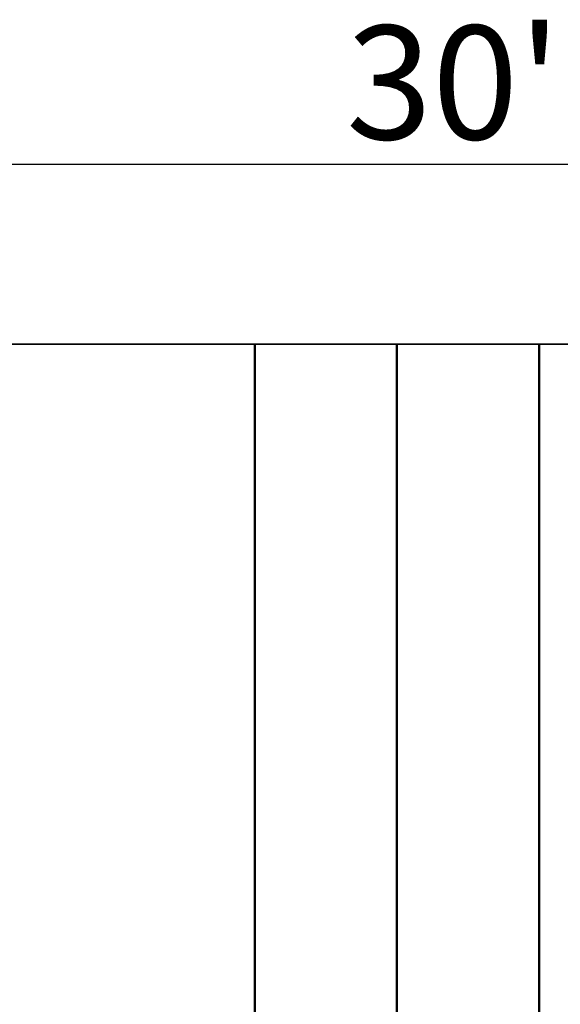
# Model space of a CAD drawing. Units: inches. Extents: x 1986 to 21484, y -1816 to 2016.
# Tile 40 of 85: x 2192 to 2230, y 1854 to 1924. Entities that reach past the tile are written whole.
import ezdxf

# ---------------------------------------------------------------- set-up
doc = ezdxf.new("R2010")
doc.units = ezdxf.units.IN
for name, color, linetype, lineweight in [('A-ANNO-DIMS', 2, 'Continuous', 18), ('A-WALL', 7, 'Continuous', 50), ('C-PROP', 7, 'Continuous', 35)]:
    doc.layers.add(name, color=color, linetype=linetype, lineweight=lineweight)
doc.styles.get("Standard").update_dxf_attribs({"font": 'arial.ttf'})
doc.dimstyles.new('ISO-25', dxfattribs={"dimtxt": 8, "dimasz": 2.5, "dimexe": 1.25, "dimexo": 0.625, "dimtad": 1, "dimdec": 1, "dimlunit": 3, "dimtxsty": 'Standard', "dimcen": 2.5, "dimadec": 0, "dimazin": 0, "dimtfac": 1, "dimtdec": 1, "dimtmove": 0, "dimatfit": 3, "dimfxl": 1, "dimarcsym": 0})

# ---------------------------------------------------------------- blocks, each defined once
blk = doc.blocks.new('*D1')
at = {"layer": 'A-ANNO-DIMS', "color": 0, "lineweight": -2, "transparency": 16777216}
for p, q in [((2042.312, 1901.377), (2042.312, 1914.655)), ((2402.312, 1901.377), (2402.312, 1914.655)), ((2044.812, 1913.405), (2399.812, 1913.405))]:
    blk.add_line(p, q, dxfattribs=at)
at = {"layer": 'A-ANNO-DIMS', "color": 0, "transparency": 16777216}
for points in [[(2044.812, 1913.821), (2044.812, 1912.988), (2042.312, 1913.405)], [(2399.812, 1913.821), (2399.812, 1912.988), (2402.312, 1913.405)]]:
    blk.add_solid(points, dxfattribs=at)
at = {"layer": 'Defpoints', "color": 0, "transparency": 16777216}
for p in [(2402.312, 1913.405), (2042.312, 1900.752), (2402.312, 1900.752)]:
    blk.add_point(p, dxfattribs=at)
at = {"layer": 'A-ANNO-DIMS', "color": 0, "transparency": 16777216, "insert": (2222.312, 1918.117), "char_height": 8, "attachment_point": 5}
blk.add_mtext("30'", dxfattribs=at)

msp = doc.modelspace()

# ---------------------------------------------------------------- linework, layer by layer
at = {"layer": 'A-WALL'}
for p, q in [((2208.312, 1900.752), (2208.312, 1852.752)), ((2218.312, 1900.752), (2218.312, 1852.752)), ((2228.312, 1900.752), (2228.312, 1852.752))]:
    msp.add_line(p, q, dxfattribs=at)
at = {"layer": 'C-PROP'}
msp.add_lwpolyline([(2042.312, 1900.752), (2402.312, 1900.752), (2402.312, 1066.752), (2042.312, 1066.752)], close=True, dxfattribs=at)

# ---------------------------------------------------------------- dimensions: what is measured, and where the dimension line sits
at = {"layer": 'A-ANNO-DIMS'}
dim = msp.add_linear_dim(base=(2402.312, 1913.405), p1=(2042.312, 1900.752), p2=(2402.312, 1900.752), dimstyle='ISO-25', override={"dimclrd": 0, "dimclre": 0, "dimclrt": 0}, dxfattribs=at)
dim.commit()
dim.dimension.update_dxf_attribs({"geometry": '*D1', "text_midpoint": (2222.312, 1918.117)})

doc.saveas('drawing.dxf')
